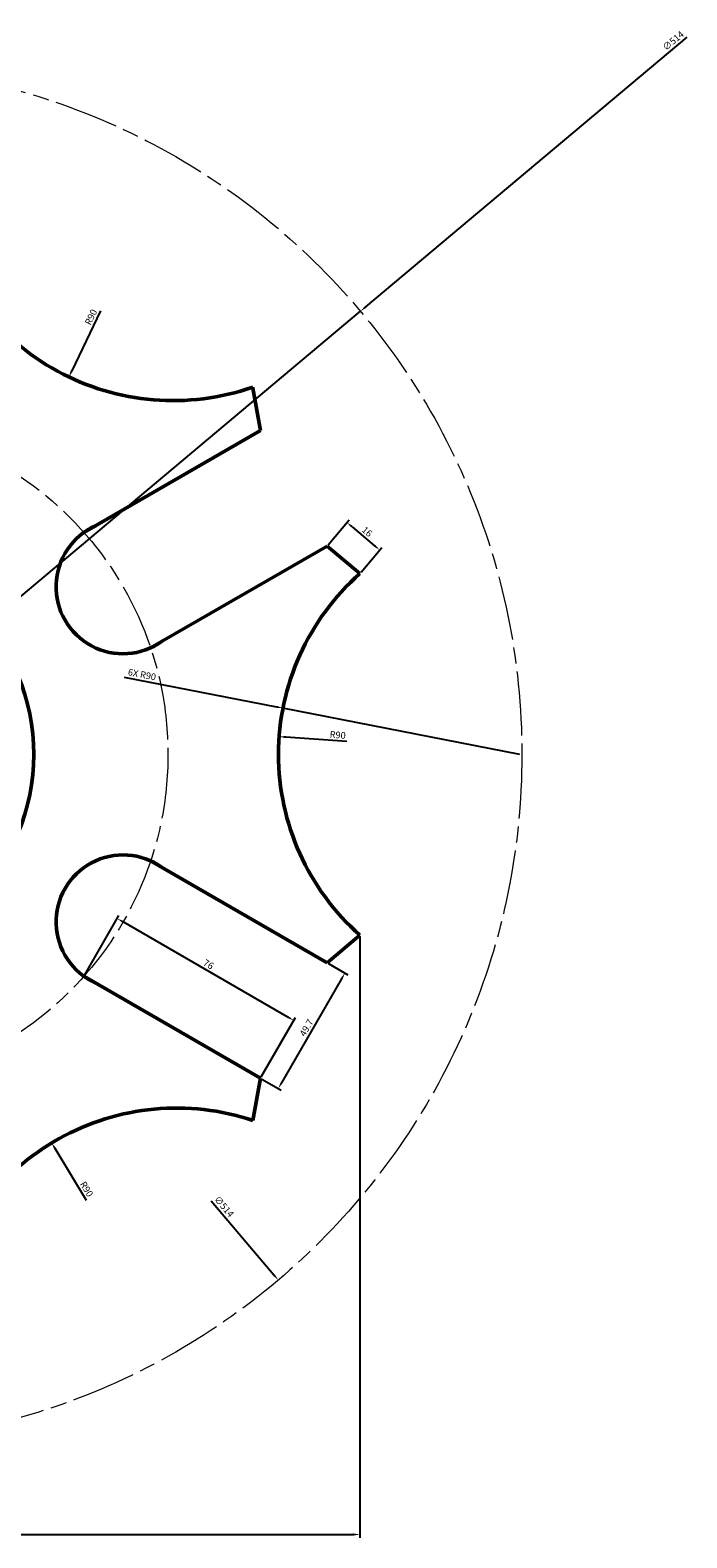
# Model space of a CAD drawing. Units: millimetres. Extents: x 1944 to 2645, y 1235 to 1798.
# Tile 3 of 3: x 2400 to 2645, y 1235 to 1798. Entities that reach past the tile are written whole.
import ezdxf

# ---------------------------------------------------------------- set-up
doc = ezdxf.new("R2010")
doc.units = ezdxf.units.MM
doc.linetypes.add('ACAD_ISO08W100', pattern=[36, 24, -3, 6, -3])
for name, color, linetype, lineweight in [('M-CONS', 8, 'ACAD_ISO08W100', 18), ('M-DIMS', 2, 'Continuous', 25), ('M-OUTL', 7, 'Continuous', 50)]:
    doc.layers.add(name, color=color, linetype=linetype, lineweight=lineweight)
doc.styles.get("Standard").update_dxf_attribs({"font": 'arial.ttf'})
doc.dimstyles.new('ISO-25', dxfattribs={"dimtxt": 2.5, "dimasz": 2.5, "dimexe": 1.25, "dimexo": 0.625, "dimtad": 1, "dimdec": 1, "dimdsep": 46, "dimtxsty": 'Standard', "dimcen": 2.5, "dimadec": 0, "dimazin": 0, "dimtfac": 1, "dimtdec": 1, "dimtmove": 0, "dimatfit": 3, "dimfxl": 1, "dimarcsym": 0})

# ---------------------------------------------------------------- blocks, each defined once
blk = doc.blocks.new('*D5')
at = {"layer": 'Defpoints', "color": 0, "lineweight": 100, "transparency": 16777216}
for p in [(2510.49, 1605.4), (2530.13, 1603.91), (2522.75, 1595.11)]:
    blk.add_point(p, dxfattribs=at)
at = {"layer": 'M-DIMS', "color": 0, "lineweight": -2, "transparency": 16777216}
for p, q in [((2510.9, 1605.88), (2518.68, 1615.15)), ((2519.79, 1612.59), (2528.22, 1605.52)), ((2523.15, 1595.59), (2530.93, 1604.87))]:
    blk.add_line(p, q, dxfattribs=at)
at = {"layer": 'M-DIMS', "color": 0, "lineweight": 100, "transparency": 16777216}
for points in [[(2520.06, 1612.91), (2519.52, 1612.27), (2517.87, 1614.19)], [(2528.48, 1605.84), (2527.95, 1605.2), (2530.13, 1603.91)]]:
    blk.add_solid(points, dxfattribs=at)
at = {"layer": 'M-DIMS', "color": 0, "transparency": 16777216, "insert": (2525.22, 1610.51), "char_height": 2.5, "attachment_point": 5, "rotation": 320}
blk.add_mtext('16', dxfattribs=at)
blk = doc.blocks.new('*D8')
at = {"layer": 'Defpoints', "color": 0, "lineweight": 100, "transparency": 16777216}
for p in [(2407.78, 1382.75), (2454.38, 1305.76)]:
    blk.add_point(p, dxfattribs=at)
at = {"layer": 'M-DIMS', "color": 0, "lineweight": -2, "transparency": 16777216}
blk.add_line((2420.77, 1361.29), (2409.07, 1380.62), dxfattribs=at)
at = {"layer": 'M-DIMS', "color": 0, "lineweight": 100, "transparency": 16777216}
blk.add_solid([(2409.43, 1380.83), (2408.71, 1380.4), (2407.78, 1382.75)], dxfattribs=at)
at = {"layer": 'M-DIMS', "color": 0, "transparency": 16777216, "insert": (2420.53, 1365.36), "char_height": 2.5, "attachment_point": 5, "rotation": 301.1863}
blk.add_mtext('R90', dxfattribs=at)
blk = doc.blocks.new('*D9')
at = {"layer": 'Defpoints', "color": 0, "lineweight": 100, "transparency": 16777216}
for p in [(2510.49, 1449.98), (2485.62, 1406.9), (2492.29, 1403.05)]:
    blk.add_point(p, dxfattribs=at)
at = {"layer": 'M-DIMS', "color": 0, "lineweight": -2, "transparency": 16777216}
for p, q in [((2511.03, 1449.67), (2518.25, 1445.51)), ((2515.91, 1443.97), (2493.54, 1405.21)), ((2486.16, 1406.59), (2493.37, 1402.42))]:
    blk.add_line(p, q, dxfattribs=at)
at = {"layer": 'M-DIMS', "color": 0, "lineweight": 100, "transparency": 16777216}
for points in [[(2515.55, 1444.18), (2516.28, 1443.76), (2517.16, 1446.13)], [(2493.18, 1405.42), (2493.9, 1405), (2492.29, 1403.05)]]:
    blk.add_solid(points, dxfattribs=at)
at = {"layer": 'M-DIMS', "color": 0, "transparency": 16777216, "insert": (2503.08, 1425.54), "char_height": 2.5, "attachment_point": 5, "rotation": 60}
blk.add_mtext('49.7', dxfattribs=at)
blk = doc.blocks.new('*D10')
at = {"layer": 'Defpoints', "color": 0, "lineweight": 100, "transparency": 16777216}
for p in [(2432.24, 1466.44), (2419.8, 1444.9), (2485.62, 1406.9)]:
    blk.add_point(p, dxfattribs=at)
at = {"layer": 'M-DIMS', "color": 0, "lineweight": -2, "transparency": 16777216}
for p, q in [((2420.11, 1445.44), (2432.86, 1467.52)), ((2495.89, 1429.69), (2434.4, 1465.19)), ((2485.93, 1407.44), (2498.68, 1429.52))]:
    blk.add_line(p, q, dxfattribs=at)
at = {"layer": 'M-DIMS', "color": 0, "lineweight": 100, "transparency": 16777216}
for points in [[(2434.61, 1465.55), (2434.19, 1464.83), (2432.24, 1466.44)], [(2496.1, 1430.05), (2495.68, 1429.33), (2498.06, 1428.44)]]:
    blk.add_solid(points, dxfattribs=at)
at = {"layer": 'M-DIMS', "color": 0, "transparency": 16777216, "insert": (2466.1, 1449.09), "char_height": 2.5, "attachment_point": 5, "rotation": 330}
blk.add_mtext('76', dxfattribs=at)
blk = doc.blocks.new('*D11')
at = {"layer": 'Defpoints', "color": 0, "lineweight": 100, "transparency": 16777216}
for p in [(2492.61, 1534.32), (2582.37, 1527.69)]:
    blk.add_point(p, dxfattribs=at)
at = {"layer": 'M-DIMS', "color": 0, "lineweight": -2, "transparency": 16777216}
blk.add_line((2517.9, 1532.45), (2495.1, 1534.13), dxfattribs=at)
at = {"layer": 'M-DIMS', "color": 0, "lineweight": 100, "transparency": 16777216}
blk.add_solid([(2495.13, 1534.55), (2495.07, 1533.72), (2492.61, 1534.32)], dxfattribs=at)
at = {"layer": 'M-DIMS', "color": 0, "transparency": 16777216, "insert": (2514.44, 1534.61), "char_height": 2.5, "attachment_point": 5, "rotation": 355.7787}
blk.add_mtext('R90', dxfattribs=at)
blk = doc.blocks.new('*D12')
at = {"layer": 'Defpoints', "color": 0, "lineweight": 100, "transparency": 16777216}
for p in [(2453.06, 1749.62), (2414.2, 1668.45)]:
    blk.add_point(p, dxfattribs=at)
at = {"layer": 'M-DIMS', "color": 0, "lineweight": -2, "transparency": 16777216}
blk.add_line((2425.99, 1693.09), (2415.28, 1670.7), dxfattribs=at)
at = {"layer": 'M-DIMS', "color": 0, "lineweight": 100, "transparency": 16777216}
blk.add_solid([(2414.9, 1670.88), (2415.65, 1670.52), (2414.2, 1668.45)], dxfattribs=at)
at = {"layer": 'M-DIMS', "color": 0, "transparency": 16777216, "insert": (2422.72, 1690.65), "char_height": 2.5, "attachment_point": 5, "rotation": 64.4138}
blk.add_mtext('R90', dxfattribs=at)
blk = doc.blocks.new('*D13')
at = {"layer": 'Defpoints', "color": 0, "lineweight": 100, "transparency": 16777216}
for p in [(2160.02, 1723.78), (2492.28, 1331.61)]:
    blk.add_point(p, dxfattribs=at)
at = {"layer": 'M-DIMS', "color": 0, "lineweight": -2, "transparency": 16777216}
blk.add_line((2467.27, 1361.13), (2490.67, 1333.51), dxfattribs=at)
at = {"layer": 'M-DIMS', "color": 0, "lineweight": 100, "transparency": 16777216}
blk.add_solid([(2490.98, 1333.78), (2490.35, 1333.24), (2492.28, 1331.61)], dxfattribs=at)
at = {"layer": 'M-DIMS', "color": 0, "transparency": 16777216, "insert": (2471.84, 1358.79), "char_height": 2.5, "attachment_point": 5, "rotation": 310.2727}
blk.add_mtext('∅514', dxfattribs=at)
blk = doc.blocks.new('GENEVA-RADIAL-SLOT-R25')
for p, q in [((0.13, 76), (0.13, 0)), ((49.87, 76), (49.87, 0))]:
    blk.add_line(p, q)
blk.add_arc((25, 73.5), 25, 354.2608, 185.7392)
blk = doc.blocks.new('*D17')
at = {"layer": 'Defpoints', "color": 0, "lineweight": 100, "transparency": 16777216}
for p in [(2129.55, 1460.27), (2522.75, 1460.27), (2522.75, 1236.69)]:
    blk.add_point(p, dxfattribs=at)
at = {"layer": 'M-DIMS', "color": 0, "lineweight": -2, "transparency": 16777216}
for p, q in [((2129.55, 1459.64), (2129.55, 1235.44)), ((2522.75, 1459.64), (2522.75, 1235.44)), ((2132.05, 1236.69), (2520.25, 1236.69))]:
    blk.add_line(p, q, dxfattribs=at)
at = {"layer": 'M-DIMS', "color": 0, "lineweight": 100, "transparency": 16777216}
for points in [[(2132.05, 1237.11), (2132.05, 1236.27), (2129.55, 1236.69)], [(2520.25, 1237.11), (2520.25, 1236.27), (2522.75, 1236.69)]]:
    blk.add_solid(points, dxfattribs=at)
at = {"layer": 'M-DIMS', "color": 0, "transparency": 16777216, "insert": (2326.15, 1238.59), "char_height": 2.5, "attachment_point": 5}
blk.add_mtext('393.2', dxfattribs=at)
blk = doc.blocks.new('*D18')
at = {"layer": 'Defpoints', "color": 0, "lineweight": 100, "transparency": 16777216}
for p in [(2522.96, 1692.97), (2129.34, 1362.42)]:
    blk.add_point(p, dxfattribs=at)
at = {"layer": 'M-DIMS', "color": 0, "lineweight": -2, "transparency": 16777216}
for p, q in [((2644.67, 1795.18), (2524.87, 1694.57)), ((2129.34, 1362.42), (2522.96, 1692.97)), ((2127.43, 1360.81), (2125.51, 1359.2))]:
    blk.add_line(p, q, dxfattribs=at)
at = {"layer": 'M-DIMS', "color": 0, "lineweight": 100, "transparency": 16777216}
for points in [[(2524.61, 1694.89), (2525.14, 1694.25), (2522.96, 1692.97)], [(2127.16, 1361.13), (2127.69, 1360.49), (2129.34, 1362.42)]]:
    blk.add_solid(points, dxfattribs=at)
at = {"layer": 'M-DIMS', "color": 0, "transparency": 16777216, "insert": (2639.78, 1793.64), "char_height": 2.5, "attachment_point": 5, "rotation": 40.0225}
blk.add_mtext('∅514', dxfattribs=at)
blk = doc.blocks.new('*D19')
at = {"layer": 'Defpoints', "color": 0, "lineweight": 100, "transparency": 16777216}
for p in [(2494.03, 1544.93), (2582.37, 1527.69)]:
    blk.add_point(p, dxfattribs=at)
at = {"layer": 'M-DIMS', "color": 0, "lineweight": -2, "transparency": 16777216}
for p, q in [((2434.85, 1556.48), (2491.58, 1545.41)), ((2582.37, 1527.69), (2494.03, 1544.93))]:
    blk.add_line(p, q, dxfattribs=at)
at = {"layer": 'M-DIMS', "color": 0, "lineweight": 100, "transparency": 16777216}
blk.add_solid([(2491.66, 1545.82), (2491.5, 1545), (2494.03, 1544.93)], dxfattribs=at)
at = {"layer": 'M-DIMS', "color": 0, "transparency": 16777216, "insert": (2441.4, 1557.14), "char_height": 2.5, "attachment_point": 5, "rotation": 348.9558}
blk.add_mtext('6X R90', dxfattribs=at)

msp = doc.modelspace()

# ---------------------------------------------------------------- linework, layer by layer
at = {"layer": 'M-CONS'}
for radius in [257, 125]:
    msp.add_circle((2326.15, 1527.69), radius, dxfattribs=at)
at = {"layer": 'M-OUTL'}
for p, q in [((2482.84, 1664.24), (2482.77, 1664.66)), ((2485.62, 1648.48), (2482.84, 1664.24)), ((2510.49, 1605.4), (2522.75, 1595.11)), ((2510.49, 1449.98), (2522.75, 1460.27)), ((2485.62, 1406.9), (2482.84, 1391.14))]:
    msp.add_line(p, q, dxfattribs=at)
msp.add_circle((2326.15, 1527.69), 75, dxfattribs=at)
for centre, start, end in [((2453.06, 1749.62), 193.4116, 289.27), ((2582.37, 1527.69), 131.4834, 228.5166), ((2454.38, 1305.76), 71.5652, 166.7342)]:
    msp.add_arc(centre, 90, start, end, dxfattribs=at)

# ---------------------------------------------------------------- block references
for p, rotation in [((2510.56, 1605.29), 119.9999999999994), ((2485.56, 1406.79), 60.00000000000047)]:
    msp.add_blockref('GENEVA-RADIAL-SLOT-R25', p, dxfattribs=dict(at, rotation=rotation))

# ---------------------------------------------------------------- dimensions: what is measured, and where the dimension line sits
at = {"layer": 'M-DIMS'}
for p1, p2, override, picture, middle in [((2129.34, 1362.42), (2522.96, 1692.97), {"dimdec": 0, "dimlfac": 1, "dimrnd": 0, "dimzin": 0, "dimdsep": 46, "dimlunit": 2}, '*D18', (2641.04, 1792.13)), ((2160.02, 1723.78), (2492.28, 1331.61), {"dimclrd": 0, "dimclre": 0, "dimclrt": 0}, '*D13', (2470.33, 1357.51))]:
    dim = msp.add_diameter_dim_2p(p1=p1, p2=p2, dimstyle='ISO-25', override=override, dxfattribs=at)
    dim.commit()
    dim.dimension.update_dxf_attribs({"geometry": picture, "text_midpoint": middle, "dimtype": 163})
for center, mpoint, picture, middle in [((2453.06, 1749.62), (2414.2, 1668.45), '*D12', (2424.43, 1689.83)), ((2582.37, 1527.69), (2492.61, 1534.32), '*D11', (2514.3, 1532.72)), ((2454.38, 1305.76), (2407.78, 1382.75), '*D8', (2418.9, 1364.37))]:
    dim = msp.add_radius_dim(center=center, mpoint=mpoint, dimstyle='ISO-25', override={"dimclrd": 0, "dimclre": 0, "dimclrt": 0}, dxfattribs=at)
    dim.commit()
    dim.dimension.update_dxf_attribs({"geometry": picture, "text_midpoint": middle, "dimtype": 164})
for p1, p2, distance, picture, middle in [((2510.49, 1605.4), (2522.75, 1595.11), 11.48, '*D5', (2525.22, 1610.51)), ((2485.62, 1406.9), (2419.8, 1444.9), -24.87, '*D10', (2466.1, 1449.09)), ((2510.49, 1449.98), (2485.62, 1406.9), 7.7, '*D9', (2503.08, 1425.54))]:
    dim = msp.add_aligned_dim(p1=p1, p2=p2, distance=distance, dimstyle='ISO-25', override={"dimclrd": 0, "dimclre": 0, "dimclrt": 0}, dxfattribs=at)
    dim.commit()
    dim.dimension.update_dxf_attribs({"geometry": picture, "text_midpoint": middle})
dim = msp.add_radius_dim(center=(2582.37, 1527.69), mpoint=(2494.03, 1544.93), text='6X <>', dimstyle='ISO-25', override={"dimdec": 0, "dimlfac": 1, "dimrnd": 0, "dimzin": 0, "dimdsep": 46, "dimlunit": 2}, dxfattribs=at)
dim.commit()
dim.dimension.update_dxf_attribs({"geometry": '*D19', "text_midpoint": (2441.03, 1555.28), "dimtype": 164})
dim = msp.add_linear_dim(base=(2522.75, 1236.69), p1=(2129.55, 1460.27), p2=(2522.75, 1460.27), dimstyle='ISO-25', override={"dimdec": 1, "dimlfac": 1, "dimrnd": 0, "dimzin": 0, "dimdsep": 46, "dimlunit": 2}, dxfattribs=at)
dim.commit()
dim.dimension.update_dxf_attribs({"geometry": '*D17', "text_midpoint": (2326.15, 1238.59)})

doc.saveas('drawing.dxf')
